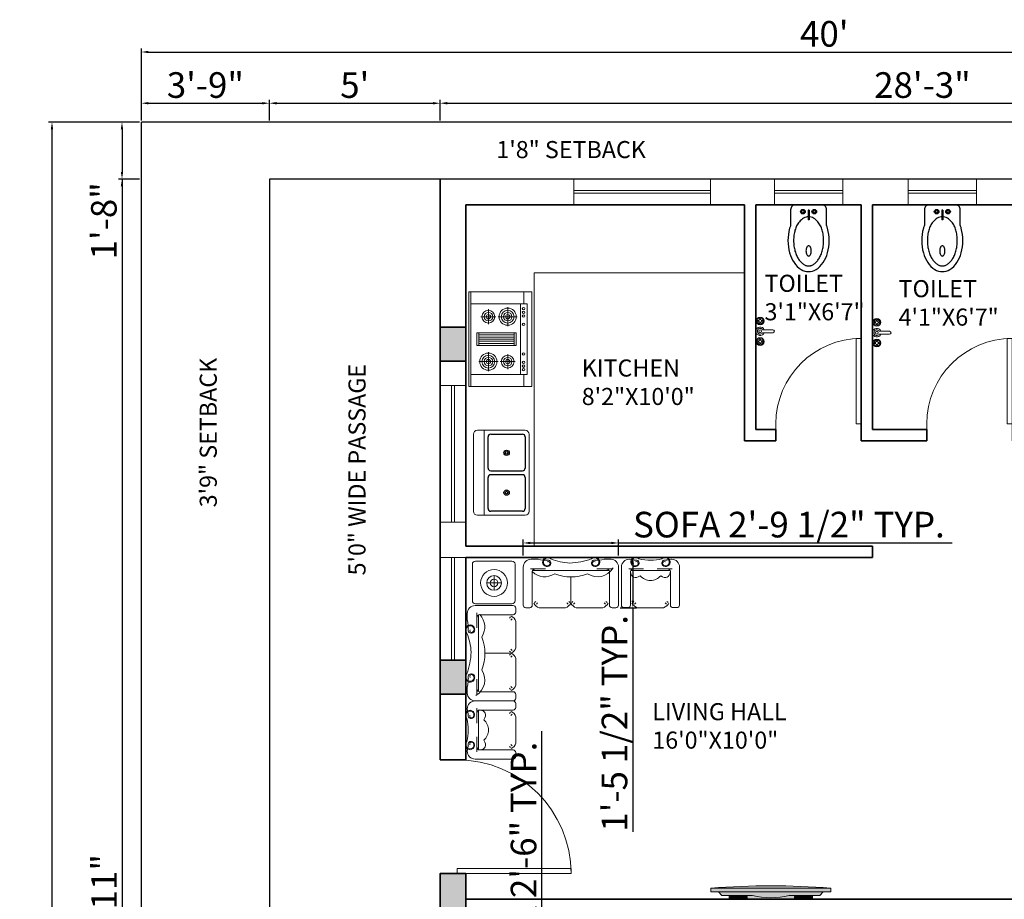
# Model space of a CAD drawing. Units: inches. Extents: x 3321 to 5237, y 11 to 1752.
# Tile 22 of 43: x 3979 to 4325, y 1434 to 1743. Entities that reach past the tile are written whole.
import ezdxf

# ---------------------------------------------------------------- set-up
doc = ezdxf.new("R2010")
doc.units = ezdxf.units.IN
for name, color, linetype, lineweight in [('A-ANNO-DIMS', 2, 'Continuous', 18), ('A-ANNO-TEXT', 7, 'Continuous', 18), ('A-AREA-IDEN', 7, 'Continuous', 18), ('A-COLS', 1, 'Continuous', 35), ('A-DOOR', 4, 'Continuous', 18), ('A-EQPM', 8, 'Continuous', 18), ('A-FLOR-CASE', 8, 'Continuous', 18), ('A-FLOR-EDGE', 7, 'Continuous', 25), ('A-GLAZ', 5, 'Continuous', 18), ('A-WALL', 7, 'Continuous', 35), ('C-PROP', 7, 'Continuous', 30), ('FUR', 42, 'Continuous', 18), ('KITSHEN', 44, 'Continuous', 18), ('moveis', 254, 'Continuous', 5), ('parede', 7, 'Continuous', 30), ('Сантехника', 7, 'Continuous', 18)]:
    doc.layers.add(name, color=color, linetype=linetype, lineweight=lineweight)
doc.layers.add('furn', color=17, linetype='Continuous')
doc.layers.add('SANTEH', color=7, linetype='Continuous')
doc.styles.get("Standard").update_dxf_attribs({"font": 'arial.ttf'})
doc.dimstyles.new('ISO-25', dxfattribs={"dimtxt": 9, "dimasz": 2.5, "dimexe": 1.25, "dimexo": 0.625, "dimtad": 1, "dimdec": 1, "dimlunit": 3, "dimtxsty": 'Standard', "dimcen": 2.5, "dimclrd": 4, "dimclre": 4, "dimclrt": 256, "dimadec": 0, "dimazin": 0, "dimtfac": 1, "dimtdec": 1, "dimtmove": 0, "dimatfit": 3, "dimfxl": 1, "dimarcsym": 0})

# ---------------------------------------------------------------- blocks, each defined once
blk = doc.blocks.new('*U2')
for p, q in [((0, 0), (0, -6)), ((-40, 0), (-40, -6))]:
    blk.add_line(p, q)
blk.add_lwpolyline([(0, 0), (0, 40), (-1.75, 40), (-1.75, 0)], close=True)
blk.add_arc((0, 0), 40, 90, 180)
blk = doc.blocks.new('*U5')
for p, q in [((0, 0), (0, -6)), ((-30, 0), (-30, -6))]:
    blk.add_line(p, q)
blk.add_lwpolyline([(0, 0), (0, 30), (-1.75, 30), (-1.75, 0)], close=True)
blk.add_arc((0, 0), 30, 90, 180)
blk = doc.blocks.new('*D48')
at = {"layer": 'A-ANNO-DIMS', "color": 0, "lineweight": -2, "transparency": 16777216}
for p, q in [((4021.39, 1707.96), (4021.39, 1715.23)), ((4023.89, 1713.98), (4063.89, 1713.98)), ((4066.39, 1707.96), (4066.39, 1715.23))]:
    blk.add_line(p, q, dxfattribs=at)
at = {"layer": 'A-ANNO-DIMS', "color": 0, "transparency": 16777216}
for points in [[(4023.89, 1714.4), (4023.89, 1713.56), (4021.39, 1713.98)], [(4063.89, 1714.4), (4063.89, 1713.56), (4066.39, 1713.98)]]:
    blk.add_solid(points, dxfattribs=at)
at = {"layer": 'Defpoints', "color": 0, "transparency": 16777216}
for p in [(4066.39, 1713.98), (4021.39, 1707.34), (4066.39, 1707.34)]:
    blk.add_point(p, dxfattribs=at)
at = {"layer": 'A-ANNO-DIMS', "color": 0, "transparency": 16777216, "insert": (4043.89, 1719.2), "char_height": 9, "attachment_point": 5}
blk.add_mtext('3\'-9"', dxfattribs=at)
blk = doc.blocks.new('*D49')
at = {"layer": 'A-ANNO-DIMS', "color": 0, "lineweight": -2, "transparency": 16777216}
for p, q in [((4066.39, 1707.96), (4066.39, 1715.23)), ((4068.89, 1713.98), (4123.89, 1713.98)), ((4126.39, 1707.96), (4126.39, 1715.23))]:
    blk.add_line(p, q, dxfattribs=at)
at = {"layer": 'A-ANNO-DIMS', "color": 0, "transparency": 16777216}
for points in [[(4068.89, 1714.4), (4068.89, 1713.56), (4066.39, 1713.98)], [(4123.89, 1714.4), (4123.89, 1713.56), (4126.39, 1713.98)]]:
    blk.add_solid(points, dxfattribs=at)
at = {"layer": 'Defpoints', "color": 0, "transparency": 16777216}
for p in [(4126.39, 1713.98), (4066.39, 1707.34), (4126.39, 1707.34)]:
    blk.add_point(p, dxfattribs=at)
at = {"layer": 'A-ANNO-DIMS', "color": 0, "transparency": 16777216, "insert": (4096.39, 1719.18), "char_height": 9, "attachment_point": 5}
blk.add_mtext("5'", dxfattribs=at)
blk = doc.blocks.new('*D50')
at = {"layer": 'A-ANNO-DIMS', "color": 0, "lineweight": -2, "transparency": 16777216}
for p, q in [((4126.39, 1707.96), (4126.39, 1715.23)), ((4128.89, 1713.98), (4462.89, 1713.98)), ((4465.39, 1707.96), (4465.39, 1715.23))]:
    blk.add_line(p, q, dxfattribs=at)
at = {"layer": 'A-ANNO-DIMS', "color": 0, "transparency": 16777216}
for points in [[(4128.89, 1714.4), (4128.89, 1713.56), (4126.39, 1713.98)], [(4462.89, 1714.4), (4462.89, 1713.56), (4465.39, 1713.98)]]:
    blk.add_solid(points, dxfattribs=at)
at = {"layer": 'Defpoints', "color": 0, "transparency": 16777216}
for p in [(4465.39, 1713.98), (4126.39, 1707.34), (4465.39, 1707.34)]:
    blk.add_point(p, dxfattribs=at)
at = {"layer": 'A-ANNO-DIMS', "color": 0, "transparency": 16777216, "insert": (4295.89, 1719.2), "char_height": 9, "attachment_point": 5}
blk.add_mtext('28\'-3"', dxfattribs=at)
blk = doc.blocks.new('*D52')
at = {"layer": 'A-ANNO-DIMS', "color": 0, "lineweight": -2, "transparency": 16777216}
for p, q in [((4020.76, 1707.34), (4013.34, 1707.34)), ((4014.59, 1704.84), (4014.59, 1689.84)), ((4020.76, 1687.34), (4013.34, 1687.34)), ((4014.59, 1687.34), (4014.59, 1660.51))]:
    blk.add_line(p, q, dxfattribs=at)
at = {"layer": 'A-ANNO-DIMS', "color": 0, "transparency": 16777216}
for points in [[(4014.17, 1704.84), (4015, 1704.84), (4014.59, 1707.34)], [(4014.17, 1689.84), (4015, 1689.84), (4014.59, 1687.34)]]:
    blk.add_solid(points, dxfattribs=at)
at = {"layer": 'Defpoints', "color": 0, "transparency": 16777216}
for p in [(4021.39, 1707.34), (4014.59, 1687.34), (4021.39, 1687.34)]:
    blk.add_point(p, dxfattribs=at)
at = {"layer": 'A-ANNO-DIMS', "color": 0, "transparency": 16777216, "insert": (4009.37, 1672.67), "char_height": 9, "attachment_point": 5, "rotation": 90}
blk.add_mtext('1\'-8"', dxfattribs=at)
blk = doc.blocks.new('*D53')
at = {"layer": 'A-ANNO-DIMS', "color": 0, "lineweight": -2, "transparency": 16777216}
for p, q in [((4020.76, 1687.34), (4013.34, 1687.34)), ((4014.59, 1684.84), (4014.59, 1174.84)), ((4020.76, 1172.34), (4013.34, 1172.34))]:
    blk.add_line(p, q, dxfattribs=at)
at = {"layer": 'A-ANNO-DIMS', "color": 0, "transparency": 16777216}
for points in [[(4014.17, 1684.84), (4015, 1684.84), (4014.59, 1687.34)], [(4014.17, 1174.84), (4015, 1174.84), (4014.59, 1172.34)]]:
    blk.add_solid(points, dxfattribs=at)
at = {"layer": 'Defpoints', "color": 0, "transparency": 16777216}
for p in [(4021.39, 1687.34), (4014.59, 1172.34), (4021.39, 1172.34)]:
    blk.add_point(p, dxfattribs=at)
at = {"layer": 'A-ANNO-DIMS', "color": 0, "transparency": 16777216, "insert": (4009.44, 1429.84), "char_height": 9, "attachment_point": 5, "rotation": 90}
blk.add_mtext('42\'-11"', dxfattribs=at)
blk = doc.blocks.new('*D63')
at = {"layer": 'A-ANNO-DIMS', "color": 0, "lineweight": -2, "transparency": 16777216}
for p, q in [((4021.39, 1707.96), (4021.39, 1733.22)), ((4023.89, 1731.97), (4498.89, 1731.97)), ((4501.39, 1707.96), (4501.39, 1733.22))]:
    blk.add_line(p, q, dxfattribs=at)
at = {"layer": 'A-ANNO-DIMS', "color": 0, "transparency": 16777216}
for points in [[(4023.89, 1732.39), (4023.89, 1731.55), (4021.39, 1731.97)], [(4498.89, 1732.39), (4498.89, 1731.55), (4501.39, 1731.97)]]:
    blk.add_solid(points, dxfattribs=at)
at = {"layer": 'Defpoints', "color": 0, "transparency": 16777216}
for p in [(4501.39, 1731.97), (4021.39, 1707.34), (4501.39, 1707.34)]:
    blk.add_point(p, dxfattribs=at)
at = {"layer": 'A-ANNO-DIMS', "color": 0, "transparency": 16777216, "insert": (4261.39, 1737.19), "char_height": 9, "attachment_point": 5}
blk.add_mtext("40'", dxfattribs=at)
blk = doc.blocks.new('*D65')
at = {"layer": 'A-ANNO-DIMS', "color": 0, "lineweight": -2, "transparency": 16777216}
for p, q in [((4020.76, 1707.34), (3988.74, 1707.34)), ((3989.99, 989.84), (3989.99, 1704.84)), ((4020.76, 987.34), (3988.74, 987.34))]:
    blk.add_line(p, q, dxfattribs=at)
at = {"layer": 'A-ANNO-DIMS', "color": 0, "transparency": 16777216}
for points in [[(3989.57, 1704.84), (3990.4, 1704.84), (3989.99, 1707.34)], [(3989.57, 989.84), (3990.4, 989.84), (3989.99, 987.34)]]:
    blk.add_solid(points, dxfattribs=at)
at = {"layer": 'Defpoints', "color": 0, "transparency": 16777216}
for p in [(3989.99, 1707.34), (4021.39, 1707.34), (4021.39, 987.34)]:
    blk.add_point(p, dxfattribs=at)
at = {"layer": 'A-ANNO-DIMS', "color": 0, "transparency": 16777216, "insert": (3984.77, 1347.34), "char_height": 9, "attachment_point": 5, "rotation": 90}
blk.add_mtext("60'", dxfattribs=at)
blk = doc.blocks.new('K10-45')
at = {"layer": 'SANTEH'}
for p, q in [((-18.9, 83.4), (-18.9, 177.1)), ((-18.9, 177.1), (-8.9, 177.1)), ((-8.9, 83.4), (-8.9, 177.1)), ((-18.9, 83.4), (-8.9, 83.4))]:
    blk.add_line(p, q, dxfattribs=at)
for points in [[(160.3, 230.4, 0.023928), (169.9, 259.6, 0.067459), (186.1, 379, 0.067459), (169.9, 498.4, 0.079812), (127.5, 591.1, 0.107118), (58, 658.5, 0.139889), (-13.9, 679, 0.139889), (-85.8, 658.5, 0.107118), (-155.3, 591.1, 0.079812), (-197.7, 498.4, 0.067459), (-213.9, 379, 0.067459), (-197.7, 259.6, 0.023928), (-188.1, 230.4), (-188.1, 80.2, 0.414214), (-138.1, 30.2), (110.3, 30.2, 0.414214), (160.3, 80.2)], [(-39.4, 478.5, 0.052061), (-37.3, 458.3, 0.065919), (-32, 443.1, 0.104629), (-22.6, 431.5, 0.172287), (-13.9, 428.4, 0.172287), (-5.2, 431.5, 0.104629), (4.1, 443.1, 0.065919), (9.5, 458.3, 0.052061), (11.6, 478.5, 0.052061), (9.5, 498.7, 0.065919), (4.1, 513.9, 0.104629), (-5.2, 525.5, 0.172287), (-13.9, 528.6, 0.172287), (-22.6, 525.5, 0.104629), (-32, 513.9, 0.065919), (-37.3, 498.7, 0.052061)]]:
    blk.add_lwpolyline(points, format="xyb", close=True, dxfattribs=at)
blk.add_lwpolyline([(-3.9, 147), (-1.4, 147.2), (10.9, 150.3), (23, 155.1), (34.7, 161.4), (45.9, 168.8), (56.5, 177.2), (66.3, 186.2), (75.2, 195.5), (83.2, 205), (90.3, 214.7), (96.5, 224.5), (102, 234.5), (106.9, 244.7), (111.1, 255.3), (114.8, 266.2), (118.1, 277.6), (121.1, 289.3), (123.7, 301.4), (126, 313.8), (127.9, 326.5), (129.3, 339.5), (130.4, 352.6), (131.1, 365.8), (131.3, 379), (131.1, 392.2), (130.4, 405.4), (129.3, 418.5), (127.9, 431.4), (126, 444.2), (123.7, 456.6), (121.1, 468.7), (118.1, 480.4), (114.8, 491.7), (111.2, 502.6), (107.3, 513.1), (103, 523.1), (98.4, 532.7), (93.5, 541.9), (88.3, 550.7), (82.8, 559.1), (77.1, 567.1), (71, 574.6), (64.9, 581.7), (58.5, 588.3), (52.1, 594.4), (45.7, 600), (39.3, 605), (33, 609.4), (26.9, 613.2), (20.8, 616.4), (14.9, 619), (9, 621.1), (3.2, 622.7), (-2.5, 623.8), (-8.2, 624.5), (-13.9, 624.7), (-19.6, 624.5), (-25.3, 623.8), (-31, 622.7), (-36.8, 621.1), (-42.7, 619), (-48.6, 616.4), (-54.7, 613.2), (-60.9, 609.4), (-67.2, 605), (-73.5, 600), (-80, 594.4), (-86.4, 588.3), (-92.7, 581.7), (-98.9, 574.6), (-104.9, 567.1), (-110.6, 559.1), (-116.1, 550.7), (-121.3, 541.9), (-126.2, 532.7), (-130.8, 523.1), (-135.1, 513.1), (-139, 502.6), (-142.7, 491.7), (-146, 480.4), (-148.9, 468.7), (-151.5, 456.6), (-153.8, 444.2), (-155.7, 431.4), (-157.2, 418.5), (-158.2, 405.4), (-158.9, 392.2), (-159.1, 379), (-158.9, 365.8), (-158.2, 352.6), (-157.2, 339.5), (-155.7, 326.5), (-153.8, 313.8), (-151.5, 301.4), (-148.9, 289.3), (-146, 277.6), (-142.6, 266.2), (-138.9, 255.3), (-134.7, 244.7), (-129.8, 234.5), (-124.4, 224.5), (-118.1, 214.7), (-111, 205), (-103.1, 195.5), (-94.1, 186.2), (-84.3, 177.2), (-73.7, 168.8), (-62.5, 161.4), (-50.8, 155.1), (-38.7, 150.3), (-26.4, 147.2), (-23.9, 147)], dxfattribs=at)
for centre, radius in [((-69.2, 98.1), 22.4), ((-69.2, 98.1), 12.4), ((41.4, 98.1), 22.4), ((41.4, 98.1), 12.4)]:
    blk.add_circle(centre, radius, dxfattribs=at)
blk = doc.blocks.new('Faucet - Bathroom top')
for p, q in [((-4.107, 0.125), (-4.375, 0.125)), ((-3.75, 0.4788), (-3.75, 0.75)), ((-3.5, 0.482), (-3.5, 0.75)), ((-3.1461, 0.125), (-2.875, 0.125)), ((3.143, 0.125), (2.875, 0.125)), ((3.5, 0.4788), (3.5, 0.75)), ((3.75, 0.482), (3.75, 0.75)), ((4.1039, 0.125), (4.375, 0.125)), ((-4.1039, -0.125), (-4.375, -0.125)), ((-3.75, -0.4821), (-3.75, -0.75)), ((-3.5, -0.4789), (-3.5, -0.75)), ((-3.143, -0.125), (-2.875, -0.125)), ((-0.5, -0.8639), (-0.5, -4.5)), ((0.5, -4.5), (0.5, -0.8631)), ((3.1461, -0.125), (2.875, -0.125)), ((3.5, -0.4821), (3.5, -0.75)), ((3.75, -0.4789), (3.75, -0.75)), ((4.107, -0.125), (4.375, -0.125))]:
    blk.add_line(p, q)
for centre, radius in [((-3.625, 0), 1.375), ((-4.625, 0), 0.2795), ((-3.625, 0), 0.5), ((-3.625, 1), 0.2795), ((-2.625, 0), 0.2795), ((0, 0), 0.5), ((3.625, 0), 1.375), ((2.625, 0), 0.2795), ((3.625, 0), 0.5), ((3.625, 1), 0.2795), ((4.625, 0), 0.2795), ((-3.625, -1), 0.2795), ((3.625, -1), 0.2795)]:
    blk.add_circle(centre, radius)
for centre, radius, start, end in [((-3.625, 0), 1, 105.2407, 164.2093), ((-3.625, 0), 1, 16.44125, 74.07887), ((0, 0), 1.5, 289.6514, 250.3603), ((0, 0), 1, 300.3431, 239.7554), ((3.625, 0), 1, 106.12, 164.0884), ((3.625, 0), 1, 16.23422, 73.90469), ((-3.625, 0), 1, 196.2342, 253.9047), ((-3.625, 0), 1, 286.12, 344.0884), ((3.625, 0), 1, 196.4413, 254.0789), ((3.625, 0), 1, 285.2407, 344.2093), ((0, -4.5), 0.5, 180, 0)]:
    blk.add_arc(centre, radius, start, end)
blk = doc.blocks.new('Oven Pln 001')
at = {"layer": 'KITSHEN'}
for p, q in [((2216.81, 1000.71), (2306.76, 1000.71)), ((2216.81, 942.71), (2216.81, 1000.71)), ((2228.09, 996.24), (2295.48, 996.24)), ((2228.09, 942.71), (2228.09, 996.24)), ((2295.48, 996.24), (2295.48, 942.71)), ((2306.76, 942.71), (2306.76, 1000.71)), ((2228.09, 993.17), (2216.81, 993.17)), ((2228.09, 990.1), (2295.48, 990.1)), ((2240.37, 968.64), (2240.37, 987.01)), ((2295.48, 993.17), (2306.76, 993.17)), ((2231.18, 977.83), (2249.55, 977.83)), ((2255.65, 983.97), (2267.93, 983.97)), ((2257.69, 950.32), (2257.69, 983.97)), ((2259.74, 983.97), (2259.74, 950.32)), ((2261.79, 950.32), (2261.79, 983.97)), ((2263.83, 983.97), (2263.83, 950.32)), ((2265.88, 950.32), (2265.88, 983.97)), ((2276.02, 977.83), (2290.39, 977.83)), ((2283.21, 970.64), (2283.21, 985.01)), ((2283.21, 950.22), (2283.21, 968.59)), ((2233.18, 959.41), (2247.55, 959.41)), ((2240.37, 952.22), (2240.37, 966.59)), ((2274.02, 959.41), (2292.39, 959.41)), ((2267.93, 950.32), (2255.65, 950.32)), ((2216.81, 940.71), (2216.81, 942.71)), ((2306.76, 942.71), (2216.81, 942.71)), ((2306.76, 940.71), (2216.81, 940.71)), ((2306.76, 940.71), (2306.76, 942.71))]:
    blk.add_line(p, q, dxfattribs=at)
blk.add_lwpolyline([(2255.65, 948.27), (2255.65, 986.01), (2267.93, 986.01), (2267.93, 948.27)], close=True, dxfattribs=at)
for centre, radius in [((2232.63, 992.94), 1.16), ((2240.37, 977.83), 8.19), ((2236.1, 992.94), 1.16), ((2239.71, 992.94), 1.16), ((2247.66, 992.94), 1.16), ((2275.92, 992.94), 1.16), ((2283.87, 992.94), 1.16), ((2287.48, 992.94), 1.16), ((2290.95, 992.94), 1.16), ((2240.37, 977.83), 6.14), ((2240.37, 977.83), 4.09), ((2240.37, 977.83), 2.05), ((2283.21, 977.83), 6.14), ((2283.21, 977.83), 4.09), ((2283.21, 977.83), 2.05), ((2283.21, 959.41), 8.19), ((2240.37, 959.41), 6.14), ((2240.37, 959.41), 4.09), ((2240.37, 959.41), 2.05), ((2283.21, 959.41), 6.14), ((2283.21, 959.41), 4.09), ((2283.21, 959.41), 2.05)]:
    blk.add_circle(centre, radius, dxfattribs=at)
blk = doc.blocks.new('ps sin 19')
at = {"layer": 'furn'}
for p, q in [((5312.25, 277.71), (5312.25, 306.28)), ((5314.63, 308.66), (5342.61, 308.66)), ((5344.99, 277.71), (5344.99, 306.28)), ((5348.56, 306.28), (5348.56, 277.71)), ((5350.94, 308.66), (5378.92, 308.66)), ((5381.3, 306.28), (5381.3, 277.71)), ((5342.61, 275.33), (5314.63, 275.33)), ((5378.92, 275.33), (5350.94, 275.33))]:
    blk.add_line(p, q, dxfattribs=at)
for centre, radius in [((5328.92, 291.99), 2.38), ((5328.92, 291.99), 1.19), ((5364.63, 291.99), 2.38), ((5364.63, 291.99), 1.19)]:
    blk.add_circle(centre, radius, dxfattribs=at)
for centre, start, end in [((5314.63, 306.28), 90, 180), ((5342.61, 306.28), 0, 90), ((5350.94, 306.28), 90, 180), ((5378.92, 306.28), 0, 90), ((5314.63, 277.71), 180, 270), ((5342.61, 277.71), 270, 0), ((5350.94, 277.71), 180, 270), ((5378.92, 277.71), 270, 0)]:
    blk.add_arc(centre, 2.38, start, end, dxfattribs=at)
at = {"layer": 'KITSHEN'}
for p, q in [((5308.68, 275.33), (5308.68, 318.18)), ((5312.25, 321.76), (5381.3, 321.76)), ((5384.87, 318.18), (5384.87, 275.33)), ((5308.68, 312.23), (5384.87, 312.23)), ((5381.3, 271.76), (5312.25, 271.76))]:
    blk.add_line(p, q, dxfattribs=at)
for centre, start, end in [((5312.25, 318.18), 90, 180), ((5381.3, 318.18), 0, 90), ((5312.25, 275.33), 180, 270), ((5381.3, 275.33), 270, 0)]:
    blk.add_arc(centre, 3.57, start, end, dxfattribs=at)
blk = doc.blocks.new('sofa-34')
at = {"color": 0, "linetype": 'ByBlock'}
for p, q in [((-0.15, 0.15), (-0.15, 0.874)), ((-0.026, 0.924), (-0.1, 0.924)), ((0.024, 0.236), (0.024, 0.874)), ((0.05, 0.838), (0.05, 0.838)), ((0.09, 0.806), (0.068, 0.824)), ((0.101, 0.857), (0.126, 0.829)), ((0.657, 0.925), (0.153, 0.925)), ((0.71, 0.857), (0.684, 0.829)), ((0.72, 0.806), (0.742, 0.824)), ((0.76, 0.838), (0.76, 0.838)), ((0.76, 0.838), (0.76, 0.838)), ((0.786, 0.236), (0.786, 0.874)), ((0.836, 0.924), (0.91, 0.924)), ((0.96, 0.15), (0.96, 0.874)), ((0.029, 0.214), (0.781, 0.214)), ((-0.01, 0.18), (0.274, 0.18)), ((0.82, 0.18), (0.536, 0.18))]:
    blk.add_line(p, q, dxfattribs=at)
blk.add_arc((0.405, 0.148), 0.258, 40.7983, 139.2017, dxfattribs=at)
at = {"color": 0, "linetype": 'ByBlock', "extrusion": (0, 0, -1)}
for centre, major_axis, ratio, start_param, end_param in [((-0.1, 0.874), (0.0354, 0.0354), 1, 3.926992, 5.497787), ((-0.026, 0.874), (-0.0354, 0.0354), 1, 0.785398, 2.356196), ((0.2, 0.766), (0.117, 0.117), 1, 4.372209, 5.213218), ((0.61, 0.766), (0.117, 0.117), 1, -0.500829, 0.34018), ((0.5, -0.587), (-0.415, 0.931), 0.264583, -0.381915, 0.387685), ((0.074, 0.236), (-0.0354, 0.0354), 1, 3.926991, 5.497788), ((0, 0.15), (0.106, 0.106), 1, 2.356194, 3.926992), ((0.179, -0.658), (-0.251, 0.635), 0.885019, 0.124301, 0.339591), ((0.117, 0.052), (-0.0624, 0.0624), 1, 4.675944, 7.152385), ((0.13, 0.052), (-0.059, 0.059), 1, 3.186406, 6.094039), ((0.114, 0.063), (-0.0458, 0.0458), 1, 6.094039, 8.043134), ((0.129, 0.073), (-0.0414, 0.0414), 1, 2.230507, 4.423483), ((0.139, 0.08), (0.0245, 0.0245), 1, 0.189152, 2.952444), ((0.118, 0.071), (0.0491, 0.0491), 1, -0.701597, 0.659711), ((0.352, -0.558), (0.735, 0.107), 0.76838, 4.597815, 5.20076)]:
    blk.add_ellipse(centre, major_axis=major_axis, ratio=ratio, start_param=start_param, end_param=end_param, dxfattribs=at)
at = {"color": 0, "linetype": 'ByBlock'}
for centre, major_axis, ratio, start_param, end_param in [((0.836, 0.874), (0.0354, 0.0354), 1, 0.785398, 2.356196), ((0.91, 0.874), (-0.0354, 0.0354), 1, 3.926992, 5.497787), ((0.31, -0.587), (0.415, 0.931), 0.264583, -0.381915, 0.387685), ((0.736, 0.236), (0.0354, 0.0354), 1, 3.926991, 5.497788), ((0.681, 0.073), (0.0414, 0.0414), 1, 2.230507, 4.423483), ((0.692, 0.071), (-0.0491, 0.0491), 1, -0.701597, 0.659711), ((0.68, 0.052), (0.059, 0.059), 1, 3.186406, 6.094039), ((0.671, 0.08), (-0.0245, 0.0245), 1, 0.189152, 2.952444), ((0.696, 0.063), (0.0458, 0.0458), 1, 6.094039, 8.043134), ((0.631, -0.658), (0.251, 0.635), 0.885019, 0.124301, 0.339591), ((0.693, 0.052), (0.0624, 0.0624), 1, 4.675944, 7.152385), ((0.81, 0.15), (-0.106, 0.106), 1, 2.356194, 3.926992)]:
    blk.add_ellipse(centre, major_axis=major_axis, ratio=ratio, start_param=start_param, end_param=end_param, dxfattribs=at)
blk = doc.blocks.new('sofa-33')
at = {"color": 0, "linetype": 'ByBlock'}
for p, q in [((-0.15, 0.15), (-0.15, 0.874)), ((-0.026, 0.924), (-0.1, 0.924)), ((0.024, 0.236), (0.024, 0.874)), ((0.05, 0.838), (0.05, 0.838)), ((0.09, 0.806), (0.068, 0.824)), ((0.101, 0.857), (0.126, 0.829)), ((0.657, 0.925), (0.153, 0.925)), ((0.71, 0.857), (0.684, 0.829)), ((0.72, 0.806), (0.742, 0.824)), ((0.76, 0.838), (0.76, 0.336)), ((0.76, 0.838), (0.76, 0.838)), ((0.76, 0.838), (0.76, 0.838)), ((0.8, 0.806), (0.778, 0.824)), ((0.811, 0.857), (0.837, 0.829)), ((0.863, 0.925), (1.367, 0.925)), ((1.42, 0.857), (1.394, 0.829)), ((1.43, 0.806), (1.452, 0.824)), ((1.47, 0.838), (1.47, 0.838)), ((1.47, 0.838), (1.47, 0.838)), ((1.496, 0.236), (1.496, 0.874)), ((1.62, 0.924), (1.546, 0.924)), ((1.67, 0.15), (1.67, 0.874)), ((0.029, 0.214), (1.491, 0.214)), ((-0.01, 0.18), (0.274, 0.18)), ((0, 0), (0.136, 0)), ((1.542, 0.18), (1.258, 0.18)), ((1.532, 0), (1.397, 0))]:
    blk.add_line(p, q, dxfattribs=at)
at = {"color": 0, "linetype": 'ByBlock', "extrusion": (0, 0, -1)}
for centre, major_axis, ratio, start_param, end_param in [((-0.1, 0.874), (0.0354, 0.0354), 1, 3.926992, 5.497787), ((-0.026, 0.874), (-0.0354, 0.0354), 1, 0.785398, 2.356196), ((0.2, 0.766), (0.117, 0.117), 1, 4.372209, 5.213218), ((0.61, 0.766), (0.117, 0.117), 1, -0.500829, 0.34018), ((0.91, 0.766), (0.117, 0.117), 1, 4.372209, 5.213218), ((1.321, 0.766), (-0.117, 0.117), 1, 1.069968, 1.910976), ((1.546, 0.874), (-0.0354, 0.0354), 1, 5.497786, 7.068583), ((1.62, 0.874), (0.0354, 0.0354), 1, -0.785398, 0.785398), ((1.147, -0.534), (0.2, 0.861), 0.59532, -0.502747, 0.502747), ((0.323, -0.666), (-0.093, 1), 0.551284, -0.397889, 0.397889), ((0.074, 0.236), (-0.0354, 0.0354), 1, 3.926991, 5.497788), ((0.766, -0.668), (-0.003, 1.004), 0.922365, -0.343589, 0.343589), ((1.446, 0.236), (0.0354, 0.0354), 1, 0.785397, 2.356194), ((0, 0.15), (0.106, 0.106), 1, 2.356194, 3.926992), ((0.282, -0.661), (-0.479, 0.479), 1, 0.566947, 0.842011), ((0.308, 0.052), (-0.0624, 0.0624), 1, 4.675944, 7.152385), ((0.321, 0.052), (-0.059, 0.059), 1, 3.186406, 6.094039), ((0.305, 0.063), (-0.0458, 0.0458), 1, 6.094039, 8.043134), ((0.32, 0.073), (-0.0414, 0.0414), 1, 2.230507, 4.423483), ((0.33, 0.08), (0.0245, 0.0245), 1, 0.189152, 2.952444), ((0.309, 0.071), (0.0491, 0.0491), 1, -0.701597, 0.659711), ((0.878, -1.382), (-0.323, 1.429), 0.878591, -0.144977, 0.144977), ((0.667, -1.39), (1.036, 1.036), 1, 5.547613, 5.837566), ((1.212, 0.073), (-0.0414, 0.0414), 1, 3.430501, 5.623477), ((1.223, 0.071), (-0.0491, 0.0491), 1, 5.623477, 6.984784), ((1.211, 0.052), (0.059, 0.059), 1, 0.189149, 3.096782), ((1.202, 0.08), (0.0245, 0.0245), 1, 1.759947, 4.52324), ((1.227, 0.063), (0.0458, 0.0458), 1, 4.52324, 6.472335), ((1.25, -0.661), (0.479, 0.479), 1, 5.441177, 5.716241), ((1.225, 0.052), (-0.0624, 0.0624), 1, 0.701599, 3.17804), ((1.52, 0.15), (0.106, 0.106), 1, 0.785398, 2.356194)]:
    blk.add_ellipse(centre, major_axis=major_axis, ratio=ratio, start_param=start_param, end_param=end_param, dxfattribs=at)
blk = doc.blocks.new('table-31')
at = {"color": 0, "linetype": 'ByBlock'}
for p, q in [((0.1683, 0.1952), (-0.1746, 0.1952)), ((-0.2031, 0.1666), (-0.2031, -0.1763)), ((0.1969, 0.1666), (0.1969, -0.1763)), ((-0.0689, 0), (0.0689, 0)), ((0, -0.0689), (0, 0.0689)), ((0.1683, -0.2048), (-0.1746, -0.2048))]:
    blk.add_line(p, q, dxfattribs=at)
for radius in [0.1261, 0.0689, 0.0353]:
    blk.add_circle((0, 0), radius, dxfattribs=at)
for centre, start, end in [((-0.1746, 0.1666), 90, 180), ((0.1683, 0.1666), 0, 90), ((-0.1746, -0.1763), 180, 270), ((0.1683, -0.1763), 270, 0)]:
    blk.add_arc(centre, 0.0286, start, end, dxfattribs=at)
blk = doc.blocks.new('PLASMA 2')
at = {"layer": 'moveis', "ltscale": 0.08}
h = blk.add_hatch(dxfattribs=at)
h.set_pattern_fill('_USER,_O', color=256, scale=0.008, double=1, pattern_type=0)
h.set_pattern_definition([(360, (-4.134502, -6.848382), (0, 0.008), []), (90, (-4.134502, -6.848382), (-0.008, 0), [])])
h.paths.add_polyline_path([(-0.2099, -0.0965), (-0.3623, -0.0965), (-0.3623, -0.1111), (-0.2099, -0.1111)])
h = blk.add_hatch(dxfattribs=at)
h.set_pattern_fill('_USER,_O', color=256, scale=0.008, double=1, pattern_type=0)
h.set_pattern_definition([(180, (4.134502, -6.848382), (0, 0.008), []), (90, (4.134502, -6.848382), (0.008, 0), [])])
h.paths.add_polyline_path([(0.2099, -0.0965), (0.3623, -0.0965), (0.3623, -0.1111), (0.2099, -0.1111)])
at = {"layer": 'parede', "ltscale": 0.08}
h = blk.add_hatch(color=256, dxfattribs=at)
h.dxf.hatch_style = 1
h.set_gradient(color1=(131, 136, 145), one_color=1, tint=1, name='CURVED')
h.paths.add_polyline_path([(-0.535, -0.0215), (0.535, -0.0215, 0.040195)])
h = blk.add_hatch(color=256, dxfattribs=at)
h.dxf.hatch_style = 1
h.set_gradient(color1=(131, 136, 145), color2=(0, 0, 0), one_color=1, name='CURVED')
h.paths.add_polyline_path([(0.535, -0.0215), (-0.535, -0.0215), (-0.535, -0.0553), (0.535, -0.0553)])
h = blk.add_hatch(color=256, dxfattribs=at)
h.dxf.hatch_style = 1
h.set_gradient(color1=(131, 136, 145), one_color=1, tint=1, name='CYLINDER')
h.paths.add_polyline_path([(0.4673, -0.0553), (-0.4673, -0.0553), (-0.4363, -0.0876), (-0.1636, -0.0876, 0.114423), (0.1636, -0.0876), (0.4363, -0.0876)])
h = blk.add_hatch(color=256, dxfattribs=at)
h.dxf.hatch_style = 1
h.set_gradient(color1=(131, 136, 145), color2=(0, 0, 0), one_color=1, name='CURVED')
h.paths.add_polyline_path([(0.3724, -0.0876), (0.1636, -0.0876, -0.114423), (-0.1636, -0.0876), (-0.3724, -0.0876), (-0.3724, -0.12), (0.3724, -0.12)])
h.paths.add_polyline_path([(-0.2099, -0.1111), (-0.3623, -0.1111), (-0.3623, -0.0965), (-0.2099, -0.0965)], flags=16)
h.paths.add_polyline_path([(0.2099, -0.1111), (0.2099, -0.0965), (0.3623, -0.0965), (0.3623, -0.1111)], flags=16)
at = {"layer": 'moveis', "ltscale": 0.08}
for p, q in [((-0.535, -0.0215), (-0.535, -0.0553)), ((-0.535, -0.0215), (0.535, -0.0215)), ((0.535, -0.0553), (-0.535, -0.0553)), ((-0.4673, -0.0553), (-0.4363, -0.0876)), ((-0.4363, -0.0876), (-0.1636, -0.0876)), ((-0.3724, -0.0876), (-0.3724, -0.12)), ((0.1636, -0.0876), (0.4363, -0.0876)), ((0.3724, -0.0876), (0.3724, -0.12)), ((0.4673, -0.0553), (0.4363, -0.0876)), ((0.535, -0.0553), (0.535, -0.0215)), ((-0.3724, -0.12), (0.3724, -0.12))]:
    blk.add_line(p, q, dxfattribs=at)
for points in [[(-0.3623, -0.0965), (-0.2099, -0.0965), (-0.2099, -0.1111), (-0.3623, -0.1111)], [(0.3623, -0.0965), (0.2099, -0.0965), (0.2099, -0.1111), (0.3623, -0.1111)]]:
    blk.add_lwpolyline(points, close=True, dxfattribs=at)
for centre, radius, start, end in [((0, -6.6658), 6.6658, 85.39647, 94.60353), ((0, 0.6178), 0.7242, 256.94486, 283.05514)]:
    blk.add_arc(centre, radius, start, end, dxfattribs=at)
blk = doc.blocks.new('COL-9X18-IN')
h = blk.add_hatch(color=256)
h.dxf.hatch_style = 1
h.paths.add_polyline_path([(9, 18), (0, 18), (0, 0), (9, 0)])
blk.add_lwpolyline([(0, 0), (9, 0), (9, 18), (0, 18)], close=True)
blk = doc.blocks.new('COL-9X12-FURN-PLAN')
h = blk.add_hatch(color=256)
h.dxf.hatch_style = 1
h.paths.add_polyline_path([(0, 12), (0, 0), (9, 0), (9, 12)])
blk.add_lwpolyline([(0, 0), (9, 0), (9, 12), (0, 12)], close=True)
blk = doc.blocks.new('WIN-48IN-9IN-WALL')
for p, q in [((0, 0), (0, 9)), ((48, 0), (48, 9)), ((0, 5), (48, 5)), ((0, 4), (48, 4))]:
    blk.add_line(p, q)
blk = doc.blocks.new('WIN-24IN-9IN-WALL')
for p, q in [((9, 24), (0, 24)), ((4, 24), (4, 0)), ((5, 24), (5, 0)), ((9, 0), (0, 0))]:
    blk.add_line(p, q)
blk = doc.blocks.new('WIN-36IN-9IN-WALL')
for p, q in [((9, 36), (0, 36)), ((4, 36), (4, 0)), ((5, 36), (5, 0)), ((9, 0), (0, 0))]:
    blk.add_line(p, q)
blk = doc.blocks.new('PROPERTY-40X60FT')
for p in [(480, 720), (0, 0)]:
    blk.add_line(p, (480, 0))
blk = doc.blocks.new('*D209')
at = {"layer": 'A-ANNO-DIMS', "color": 4, "lineweight": -2, "transparency": 16777216}
for p, q in [((4155.59, 1555.1), (4155.59, 1560.75)), ((4189.09, 1555.1), (4189.09, 1560.75)), ((4158.09, 1559.5), (4186.59, 1559.5)), ((4189.09, 1559.5), (4306.35, 1559.5))]:
    blk.add_line(p, q, dxfattribs=at)
at = {"layer": 'A-ANNO-DIMS', "color": 4, "transparency": 16777216}
for points in [[(4158.09, 1559.92), (4158.09, 1559.08), (4155.59, 1559.5)], [(4186.59, 1559.92), (4186.59, 1559.08), (4189.09, 1559.5)]]:
    blk.add_solid(points, dxfattribs=at)
at = {"layer": 'Defpoints', "color": 0, "transparency": 16777216}
for p in [(4189.09, 1559.5), (4155.59, 1554.48), (4189.09, 1554.48)]:
    blk.add_point(p, dxfattribs=at)
at = {"layer": 'A-ANNO-DIMS', "transparency": 16777216, "insert": (4248.97, 1564.78), "char_height": 9, "attachment_point": 5}
blk.add_mtext('SOFA 2\'-9 1/2" TYP.', dxfattribs=at)
blk = doc.blocks.new('*D210')
at = {"layer": 'A-ANNO-DIMS', "color": 4, "lineweight": -2, "transparency": 16777216}
for p, q in [((4189.71, 1554.48), (4195.36, 1554.48)), ((4194.11, 1551.98), (4194.11, 1539.24)), ((4189.71, 1536.74), (4195.36, 1536.74)), ((4194.11, 1536.74), (4194.11, 1458.01))]:
    blk.add_line(p, q, dxfattribs=at)
at = {"layer": 'A-ANNO-DIMS', "color": 4, "transparency": 16777216}
for points in [[(4193.69, 1551.98), (4194.53, 1551.98), (4194.11, 1554.48)], [(4193.69, 1539.24), (4194.53, 1539.24), (4194.11, 1536.74)]]:
    blk.add_solid(points, dxfattribs=at)
at = {"layer": 'Defpoints', "color": 0, "transparency": 16777216}
for p in [(4189.09, 1554.48), (4189.09, 1536.74), (4194.11, 1536.74)]:
    blk.add_point(p, dxfattribs=at)
at = {"layer": 'A-ANNO-DIMS', "transparency": 16777216, "insert": (4188.83, 1496.12), "char_height": 9, "attachment_point": 5, "rotation": 90}
blk.add_mtext('1\'-5 1/2" TYP.', dxfattribs=at)
blk = doc.blocks.new('*D219')
at = {"layer": 'A-ANNO-DIMS', "color": 4, "lineweight": -2, "transparency": 16777216}
for p, q in [((4162.16, 1343.6), (4162.16, 1493.33)), ((4158.31, 1343.6), (4163.41, 1343.6)), ((4162.16, 1316.25), (4162.16, 1341.1)), ((4158.31, 1313.75), (4163.41, 1313.75))]:
    blk.add_line(p, q, dxfattribs=at)
at = {"layer": 'A-ANNO-DIMS', "color": 4, "transparency": 16777216}
for points in [[(4161.74, 1341.1), (4162.58, 1341.1), (4162.16, 1343.6)], [(4161.74, 1316.25), (4162.58, 1316.25), (4162.16, 1313.75)]]:
    blk.add_solid(points, dxfattribs=at)
at = {"layer": 'Defpoints', "color": 0, "transparency": 16777216}
for p in [(4157.68, 1343.6), (4162.16, 1343.6), (4157.68, 1313.75)]:
    blk.add_point(p, dxfattribs=at)
at = {"layer": 'A-ANNO-DIMS', "transparency": 16777216, "insert": (4156.88, 1419.72), "char_height": 9, "attachment_point": 5, "rotation": 90}
blk.add_mtext('KITCHEN SINK 2\'-6" TYP.', dxfattribs=at)

msp = doc.modelspace()

# ---------------------------------------------------------------- linework, layer by layer
at = {"layer": 'A-FLOR-CASE'}
for p, q in [((4159.39, 1654.34), (4159.39, 1558.34)), ((4233.39, 1654.34), (4159.39, 1654.34))]:
    msp.add_line(p, q, dxfattribs=at)
at = {"layer": 'A-FLOR-EDGE'}
for p, q in [((4465.39, 1687.34), (4066.39, 1687.34)), ((4066.39, 1687.34), (4066.39, 1091.34))]:
    msp.add_line(p, q, dxfattribs=at)
at = {"layer": 'A-WALL'}
for p, q in [((4126.39, 1687.34), (4126.39, 1483.34)), ((4135.39, 1678.34), (4135.39, 1558.34)), ((4233.39, 1678.34), (4135.39, 1678.34)), ((4233.39, 1678.34), (4233.39, 1595.34)), ((4237.39, 1678.34), (4237.39, 1599.34)), ((4274.39, 1678.34), (4237.39, 1678.34)), ((4274.39, 1678.34), (4274.39, 1595.34)), ((4327.39, 1678.34), (4278.39, 1678.34)), ((4278.39, 1678.34), (4278.39, 1599.34)), ((4244.39, 1599.34), (4237.39, 1599.34)), ((4244.39, 1599.34), (4244.39, 1595.34)), ((4297.39, 1599.34), (4278.39, 1599.34)), ((4297.39, 1599.34), (4297.39, 1595.34)), ((4244.39, 1595.34), (4233.39, 1595.34)), ((4297.39, 1595.34), (4274.39, 1595.34)), ((4278.39, 1558.34), (4135.39, 1558.34)), ((4278.39, 1558.34), (4278.39, 1554.34)), ((4135.39, 1554.34), (4135.39, 1483.34)), ((4135.39, 1554.34), (4278.39, 1554.34)), ((4126.39, 1483.34), (4135.39, 1483.34)), ((4126.39, 1443.34), (4135.39, 1443.34)), ((4126.39, 1443.34), (4126.39, 1221.34)), ((4135.39, 1443.34), (4135.39, 1434.34)), ((4135.39, 1434.34), (4327.39, 1434.34))]:
    msp.add_line(p, q, dxfattribs=at)

# ---------------------------------------------------------------- block references
at = {"layer": 'A-COLS'}
for p in [(4126.39, 1623.34), (4126.39, 1506.34)]:
    msp.add_blockref('COL-9X12-FURN-PLAN', p, dxfattribs=at)
at = {"layer": 'A-COLS', "rotation": 180}
msp.add_blockref('COL-9X18-IN', (4135.39, 1443.34), dxfattribs=at)
at = {"layer": 'A-DOOR'}
for p in [(4274.39, 1601.34), (4327.39, 1601.34)]:
    msp.add_blockref('*U5', p, dxfattribs=at)
at = {"layer": 'A-DOOR', "rotation": 270}
msp.add_blockref('*U2', (4132.39, 1443.34), dxfattribs=at)
at = {"layer": 'A-EQPM', "xscale": 39.3701, "yscale": 39.3701, "zscale": 39.3701}
msp.add_blockref('PLASMA 2', (4242.61, 1439.06), dxfattribs=at)
at = {"layer": 'A-GLAZ'}
for name, p in [('WIN-48IN-9IN-WALL', (4173.36, 1678.34)), ('WIN-36IN-9IN-WALL', (4126.39, 1518.34))]:
    msp.add_blockref(name, p, dxfattribs=at)
for name, p, rotation in [('WIN-24IN-9IN-WALL', (4243.89, 1687.34), 269.9999999999957), ('WIN-24IN-9IN-WALL', (4290.89, 1687.34), 269.9999999999943), ('WIN-48IN-9IN-WALL', (4135.39, 1566.84), 89.99999999999824)]:
    msp.add_blockref(name, p, dxfattribs=dict(at, rotation=rotation))
at = {"layer": 'C-PROP', "rotation": 180}
msp.add_blockref('PROPERTY-40X60FT', (4501.39, 1707.34), dxfattribs=at)
at = {"layer": 'FUR'}
for name, p, xscale, yscale, zscale, rotation in [('sofa-33', (4158.35, 1553.77), -18.40353949668526, 18.40353949668526, 18.40353949668526, 180), ('sofa-34', (4192.85, 1553.78), -18.40353949668526, 18.40353949668526, 18.40353949668526, 180), ('table-31', (4145.34, 1545.45), -37.41559934897337, 37.41559934897337, 37.41559934897337, 180), ('sofa-33', (4135.95, 1534.75), 18.40353949668526, 18.40353949668526, 18.40353949668526, 270), ('sofa-34', (4135.94, 1501.25), 18.40353949668526, 18.40353949668526, 18.40353949668526, 270)]:
    msp.add_blockref(name, p, dxfattribs=dict(at, xscale=xscale, yscale=yscale, zscale=zscale, rotation=rotation))
at = {"layer": 'KITSHEN'}
for name, p, xscale, yscale, zscale, rotation in [('Oven Pln 001', (3789.74, 2464.72), 0.3685700214197002, 0.3685700214197002, 0.3685700214197002, 270), ('ps sin 19', (4264.15, -510.57), 0.3917772908061623, 0.3917772908061623, 0.3917772908061623, 90)]:
    msp.add_blockref(name, p, dxfattribs=dict(at, xscale=xscale, yscale=yscale, zscale=zscale, rotation=rotation))
at = {"layer": 'Сантехника', "xscale": 0.0362080263207385, "yscale": 0.0362080263207385, "zscale": 0.0362080263207385, "rotation": 180}
for p in [(4255.38, 1679.43), (4302.38, 1679.43)]:
    msp.add_blockref('K10-45', p, dxfattribs=at)
at = {"layer": 'Сантехника', "rotation": 90}
for p in [(4238.87, 1633.87), (4279.87, 1633.37)]:
    msp.add_blockref('Faucet - Bathroom top', p, dxfattribs=at)

# ---------------------------------------------------------------- texts
at = {"layer": 'A-ANNO-TEXT', "insert": (4146.15, 1700.7), "char_height": 6, "attachment_point": 1}
msp.add_mtext_dynamic_manual_height_columns('1\'8" SETBACK', width=97.3114, gutter_width=25, heights=[0], dxfattribs=at)
at = {"layer": 'A-ANNO-TEXT', "insert": (4041.9, 1572.02), "char_height": 6, "attachment_point": 1, "rotation": 90}
msp.add_mtext_dynamic_manual_height_columns('3\'9" SETBACK', width=97.3114, gutter_width=25, heights=[0], dxfattribs=at)
at = {"layer": 'A-AREA-IDEN', "char_height": 6, "attachment_point": 1}
for s, insert in [('TOILET\\P3\'1"X6\'7"', (4240.4, 1653.72)), ('TOILET\\P4\'1"X6\'7"', (4287.51, 1651.84)), ('KITCHEN\\P8\'2"X10\'0"', (4176.15, 1623.96)), ('LIVING HALL\\P16\'0"X10\'0"', (4200.96, 1503.23))]:
    msp.add_mtext_dynamic_manual_height_columns(s, width=97.3114, gutter_width=25, heights=[0], dxfattribs=dict(at, insert=insert))
at = {"layer": 'A-AREA-IDEN', "insert": (4094.18, 1548.09), "char_height": 6, "attachment_point": 1, "rotation": 90}
msp.add_mtext_dynamic_manual_height_columns('5\'0" WIDE PASSAGE', width=97.3114, gutter_width=25, heights=[0], dxfattribs=at)

# ---------------------------------------------------------------- dimensions: what is measured, and where the dimension line sits
at = {"layer": 'A-ANNO-DIMS'}
for base, p1, p2, override, picture, middle in [((4501.39, 1731.97), (4021.39, 1707.34), (4501.39, 1707.34), {"dimclrd": 0, "dimclre": 0, "dimclrt": 0}, '*D63', (4261.39, 1737.19)), ((4066.39, 1713.98), (4021.39, 1707.34), (4066.39, 1707.34), {"dimclrd": 0, "dimclre": 0, "dimclrt": 0}, '*D48', (4043.89, 1719.2)), ((4126.39, 1713.98), (4066.39, 1707.34), (4126.39, 1707.34), {"dimclrd": 0, "dimclre": 0, "dimclrt": 0, "dimtmove": 1}, '*D49', (4096.39, 1719.18)), ((4465.39, 1713.98), (4126.39, 1707.34), (4465.39, 1707.34), {"dimclrd": 0, "dimclre": 0, "dimclrt": 0, "dimtmove": 1}, '*D50', (4295.89, 1719.2))]:
    dim = msp.add_linear_dim(base=base, p1=p1, p2=p2, dimstyle='ISO-25', override=override, dxfattribs=at)
    dim.commit()
    dim.dimension.update_dxf_attribs({"geometry": picture, "text_midpoint": middle})
for base, p1, p2, angle, override, picture, middle in [((3989.99, 1707.34), (4021.39, 987.34), (4021.39, 1707.34), 270, {"dimclrd": 0, "dimclre": 0, "dimclrt": 0}, '*D65', (3984.77, 1347.34)), ((4014.59, 1687.34), (4021.39, 1707.34), (4021.39, 1687.34), 90, {"dimclrd": 0, "dimclre": 0, "dimclrt": 0}, '*D52', (4009.37, 1672.67)), ((4014.59, 1172.34), (4021.39, 1687.34), (4021.39, 1172.34), 90, {"dimclrd": 0, "dimclre": 0, "dimclrt": 0, "dimtmove": 1}, '*D53', (4009.44, 1429.84))]:
    dim = msp.add_linear_dim(base=base, p1=p1, p2=p2, angle=angle, dimstyle='ISO-25', override=override, dxfattribs=at)
    dim.commit()
    dim.dimension.update_dxf_attribs({"geometry": picture, "text_midpoint": middle})
dim = msp.add_linear_dim(base=(4189.09, 1559.5), p1=(4155.59, 1554.48), p2=(4189.09, 1554.48), text='SOFA <> TYP.', dimstyle='ISO-25', override={"dimdec": 1, "dimlfac": 1, "dimrnd": 0, "dimzin": 1, "dimdsep": 46, "dimlunit": 4, "dimfrac": 2}, dxfattribs=at)
dim.commit()
dim.dimension.update_dxf_attribs({"geometry": '*D209', "text_midpoint": (4248.97, 1564.78)})
for base, p1, p2, angle, text, picture, middle in [((4194.11, 1536.74), (4189.09, 1554.48), (4189.09, 1536.74), 270, '<> TYP.', '*D210', (4188.83, 1496.12)), ((4162.1594, 1343.6044), (4157.682, 1313.7547), (4157.682, 1343.6044), 90, 'KITCHEN SINK <> TYP.', '*D219', (4156.8809, 1419.7178))]:
    dim = msp.add_linear_dim(base=base, p1=p1, p2=p2, angle=angle, text=text, dimstyle='ISO-25', override={"dimdec": 1, "dimlfac": 1, "dimrnd": 0, "dimzin": 1, "dimdsep": 46, "dimlunit": 4, "dimfrac": 2}, dxfattribs=at)
    dim.commit()
    dim.dimension.update_dxf_attribs({"geometry": picture, "text_midpoint": middle})

doc.saveas('drawing.dxf')
